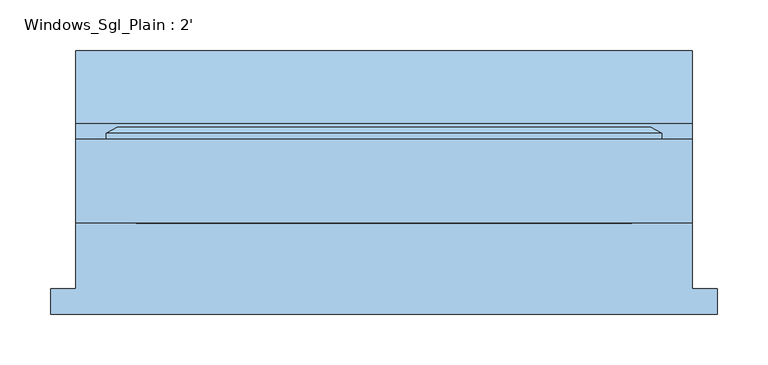
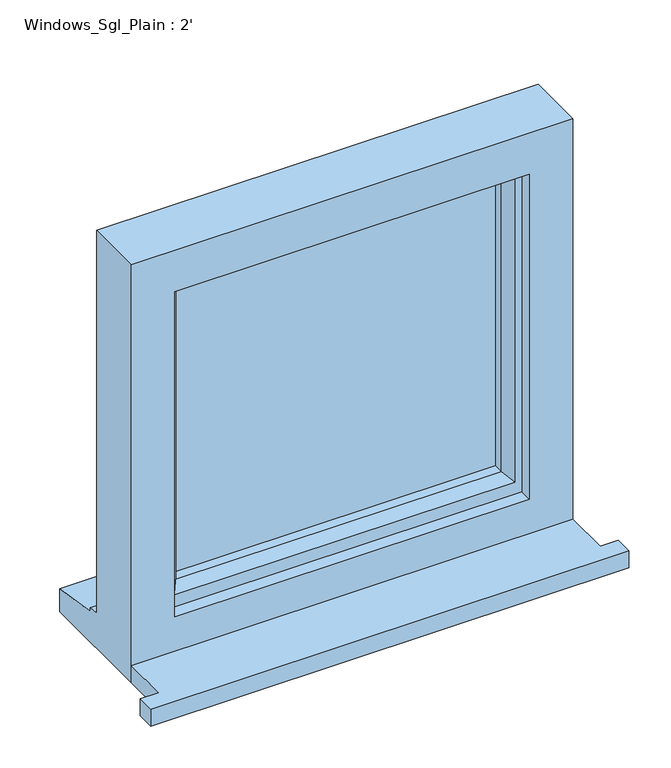
"""IFC4 building model written with IfcOpenShell, lengths in millimetres: window geometry, Windows_Sgl_Plain : 2'."""

from ifc_helpers import new_model, si_unit, frame, origin, place, context, project, spatial, polyline, outline, extrude, faceted_brep, source, transform, mapped, element, save


def windows_sgl_plain_2_82341a49(model_context):
    return source(origin(), model_context, "Body", "SolidModel", [
        extrude(outline(polyline([(-329.8, -115.6034322), (-329.8, -90.6034322), (-304.8, -90.6034322), (-304.8, -25.4834322), (304.8, -25.4834322), (304.8, -90.6034322), (329.8, -90.6034322), (329.8, -115.6034322), (-329.8, -115.6034322)])), frame((0.0, 0.0, 1500.4), z_axis=(0.0, 0.0, 1.0), x_axis=(1.0, 0.0, 0.0)), (0.0, 0.0, 1.0), 25.0),
        faceted_brep([(-304.8, -25.4834322, 1500.4), (304.8, -25.4834322, 1500.4), (304.8, -25.4834322, 2110.0), (-304.8, -25.4834322, 2110.0), (-244.8, -25.4834322, 2050.0), (244.8, -25.4834322, 2050.0), (244.8, -25.4834322, 1575.4), (-244.8, -25.4834322, 1575.4), (-304.8, 57.5165678, 2110.0), (-304.8, 57.5165678, 1551.4), (-304.8, 72.5165678, 1550.08767), (-304.8, 72.5165678, 1545.1449676), (-304.8, 145.0165678, 1534.2088847), (-304.8, 145.0165678, 1500.4), (304.8, 57.5165678, 2110.0), (304.8, 57.5165678, 1551.4), (-264.8, 57.5165678, 2070.0), (-264.8, 57.5165678, 1563.4), (264.8, 57.5165678, 1563.4), (264.8, 57.5165678, 2070.0), (-264.8, -7.4834322, 2070.0), (-264.8, -7.4834322, 1563.4), (264.8, -7.4834322, 2070.0), (264.8, -7.4834322, 1563.4), (-244.8, -7.4834322, 2050.0), (-244.8, -7.4834322, 1575.4), (244.8, -7.4834322, 1575.4), (244.8, -7.4834322, 2050.0), (304.8, 145.0165678, 1500.4), (304.8, 145.0165678, 1534.2088847), (304.8, 72.5165678, 1545.1449676), (304.8, 72.5165678, 1550.08767)], [[[0, 1, 2, 3], [4, 5, 6, 7]], [[0, 3, 8, 9, 10, 11, 12, 13]], [[9, 8, 14, 15], [16, 17, 18, 19]], [[17, 16, 20, 21]], [[20, 22, 23, 21], [24, 25, 26, 27]], [[24, 4, 7, 25]], [[3, 2, 14, 8]], [[16, 19, 22, 20]], [[5, 4, 24, 27]], [[15, 14, 2, 1, 28, 29, 30, 31]], [[19, 18, 23, 22]], [[5, 27, 26, 6]], [[28, 1, 0, 13]], [[29, 28, 13, 12]], [[30, 29, 12, 11]], [[31, 30, 11, 10]], [[15, 31, 10, 9]], [[21, 23, 18, 17]], [[7, 6, 26, 25]]]),
        extrude(outline(polyline([(234.8, 21.5165678), (-234.8, 21.5165678), (-234.8, 45.5165678), (234.8, 45.5165678), (234.8, 21.5165678)])), frame((0.0, 0.0, 1593.4), z_axis=(0.0, 0.0, 1.0), x_axis=(1.0, 0.0, 0.0)), (0.0, 0.0, 1.0), 446.6),
        faceted_brep([(-274.8, 57.5165678, 2080.0), (-274.8, 63.2900705, 2080.0), (-274.8, 63.2900705, 1553.4), (-274.8, 57.5165678, 1553.4), (-264.8, -7.4834322, 2070.0), (-264.8, 57.5165678, 2070.0), (-264.8, 57.5165678, 1563.4), (-264.8, -7.4834322, 1563.4), (-224.8, 7.0094677, 2030.0), (-234.9480377, -7.4834322, 2040.1480377), (-234.9480377, -7.4834322, 1593.2519623), (-224.8, 7.0094677, 1603.4), (-224.8, 21.5165678, 2030.0), (-224.8, 21.5165678, 1603.4), (-234.8, 45.5165678, 2040.0), (-234.8, 21.5165678, 2040.0), (-234.8, 21.5165678, 1593.4), (-234.8, 45.5165678, 1593.4), (-224.8, 63.2900705, 2030.0), (-224.8, 45.5165678, 2030.0), (-224.8, 45.5165678, 1603.4), (-224.8, 63.2900705, 1603.4), (-242.2457548, 69.0635732, 2047.4457548), (-242.2457548, 69.0635732, 1585.9542452), (-264.0153903, 69.0635732, 2069.2153903), (-264.0153903, 69.0635732, 1564.1846097), (274.8, 63.2900705, 1553.4), (274.8, 57.5165678, 1553.4), (264.8, 57.5165678, 1563.4), (264.8, -7.4834322, 1563.4), (234.9480377, -7.4834322, 1593.2519623), (224.8, 7.0094677, 1603.4), (224.8, 21.5165678, 1603.4), (234.8, 21.5165678, 1593.4), (234.8, 45.5165678, 1593.4), (224.8, 45.5165678, 1603.4), (224.8, 63.2900705, 1603.4), (242.2457548, 69.0635732, 1585.9542452), (264.0153903, 69.0635732, 1564.1846097), (274.8, 63.2900705, 2080.0), (274.8, 57.5165678, 2080.0), (264.8, 57.5165678, 2070.0), (264.8, -7.4834322, 2070.0), (234.9480377, -7.4834322, 2040.1480377), (224.8, 7.0094677, 2030.0), (224.8, 21.5165678, 2030.0), (234.8, 21.5165678, 2040.0), (234.8, 45.5165678, 2040.0), (224.8, 45.5165678, 2030.0), (224.8, 63.2900705, 2030.0), (242.2457548, 69.0635732, 2047.4457548), (264.0153903, 69.0635732, 2069.2153903)], [[[0, 1, 2, 3]], [[4, 5, 6, 7]], [[8, 9, 10, 11]], [[12, 8, 11, 13]], [[14, 15, 16, 17]], [[18, 19, 20, 21]], [[22, 18, 21, 23]], [[1, 24, 25, 2]], [[3, 2, 26, 27]], [[7, 6, 28, 29]], [[11, 10, 30, 31]], [[13, 11, 31, 32]], [[17, 16, 33, 34]], [[21, 20, 35, 36]], [[23, 21, 36, 37]], [[2, 25, 38, 26]], [[27, 26, 39, 40]], [[29, 28, 41, 42]], [[31, 30, 43, 44]], [[32, 31, 44, 45]], [[34, 33, 46, 47]], [[36, 35, 48, 49]], [[37, 36, 49, 50]], [[26, 38, 51, 39]], [[40, 39, 1, 0]], [[3, 27, 40, 0], [5, 41, 28, 6]], [[42, 41, 5, 4]], [[7, 29, 42, 4], [9, 43, 30, 10]], [[44, 43, 9, 8]], [[45, 44, 8, 12]], [[15, 46, 33, 16], [13, 32, 45, 12]], [[47, 46, 15, 14]], [[17, 34, 47, 14], [19, 48, 35, 20]], [[49, 48, 19, 18]], [[50, 49, 18, 22]], [[24, 51, 38, 25], [23, 37, 50, 22]], [[39, 51, 24, 1]]]),
    ])


if __name__ == "__main__":
    model = new_model("IFC4")
    model_context = context("Model", 3, world=origin())
    ifc_project = project(units=[si_unit("LENGTHUNIT", "METRE", prefix="MILLI")], contexts=[model_context])
    site = spatial("IfcSite", under=ifc_project)
    building = spatial("IfcBuilding", under=site)
    placement = place(None, origin())
    windows_sgl_plain_2_shape = windows_sgl_plain_2_82341a49(model_context)
    element("IfcWindow", 1, ObjectType="Windows_Sgl_Plain : 2'", at=placement, inside=building, context=model_context, shape_type="MappedRepresentation", body=[
        mapped(windows_sgl_plain_2_shape, transform((0.0, 0.0, 0.0), x_axis=(1.0, 0.0, 0.0), y_axis=(0.0, 1.0, 0.0), z_axis=(0.0, 0.0, 1.0))),
    ])
    save(model, "model.ifc")

# Revit data of these elements
# Type "Windows_Sgl_Plain : 2'"
#   Type Mark = "60"
#   Operation = "SinglePanel"
#   Construction Type Id = "SGL"
#   Manufacturer = "Revit"
#   Keynote = "L10"
#   Analytic Construction = "Large single-glazed windows"
#   Wrap Layers (Ext) from Ext = 0.336286 ft
#   Wrap Layers (Int) from Ext = 0.582349 ft
#   Window Board Projection = 0.082021 ft
#   Window Board Extension = 0.082021 ft
#   Visual Light Transmittance = 0.9
#   Solar Heat Gain Coefficient = 0.86
#   Rough Width = 2.0 ft
#   Rough Height = 2.0 ft
#   Height = 2.0 ft
#   Width = 2.0 ft
#   Heat Transfer Coefficient (U) = 5.5617 W/(m²·K)
#   Glazing Thickness = 0.07874 ft
#   FrameOffset - External = 0.164042 ft
#   Frame Depth = 0.213255 ft
#   Default Head Height = 6.922572 ft
#   Cill Depth = 0.287073 ft
#   Cavity Closer Width = 0.164042 ft
#   Cavity Closer Offset from Ext = 0.336286 ft
#   Cavity Closer Depth = 0.278871 ft
#   Vis - Cavity Closers = yes
#   Define Thermal Properties by = 1
#   Material Trim = Window Frame
#   Material Glass = Glass
#   Material Frame = Window Frame
#   Wall Closure = (empty or 0)
# Element 1 (IfcWindow, "Windows_Sgl_Plain : 2'")
#   Materials on its faces: "Window Frame", "Glass"
# Materials
#   "Window Frame": colour RGB 249 249 249, transparency 0, Keynote = "L10", Cost = 0
#   "Glass": class "Glass", colour RGB 0 128 192, transparency 0.9, Description = "Soda Lime Glass", Cost = 0
